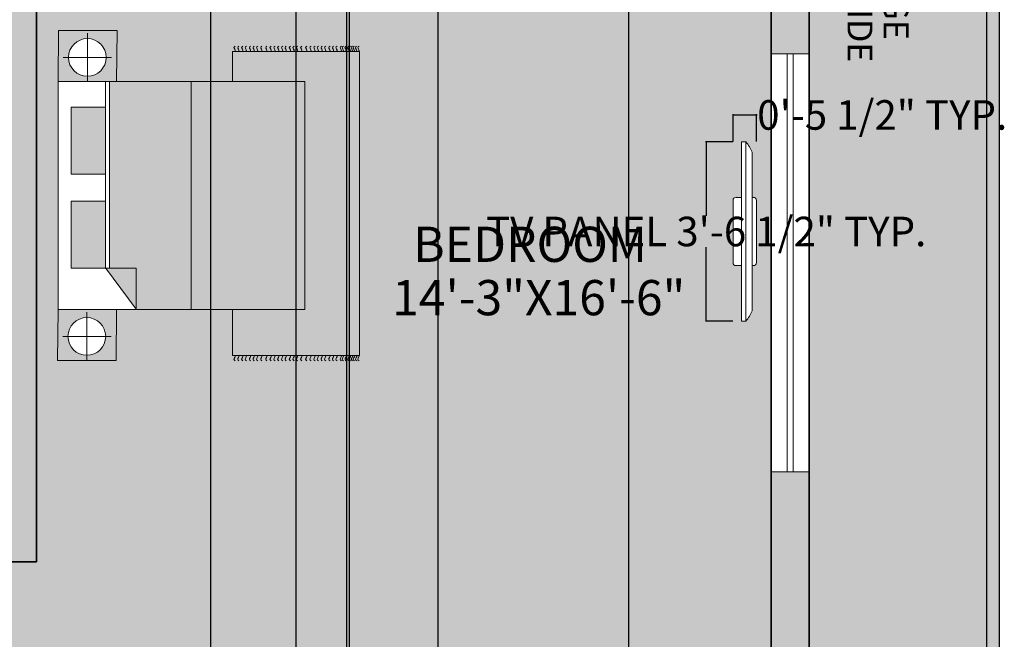
# Model space of a CAD drawing. Units: inches. Extents: x 1884 to 2398, y 474 to 1488.
# Tile 37 of 39: x 2165 to 2398, y 1087 to 1233. Entities that reach past the tile are written whole.
import ezdxf

# ---------------------------------------------------------------- set-up
doc = ezdxf.new("R2010")
doc.units = ezdxf.units.IN
doc.header["$MEASUREMENT"] = 0
for name, color, linetype, lineweight in [('A-ANNO-DIMS', 2, 'Continuous', 18), ('A-AREA-IDEN', 7, 'Continuous', 18), ('A-EQPM', 8, 'Continuous', 18), ('A-FLOR-PATT', 254, 'Continuous', 13), ('A-FURN-PATT', 253, 'Continuous', 13), ('A-WALL-PATT', 250, 'Continuous', 13), ('C-PROP', 7, 'Continuous', 30), ('furniture', 8, 'Continuous', 18), ('walls', 7, 'Continuous', 35), ('windows', 4, 'Continuous', 18)]:
    doc.layers.add(name, color=color, linetype=linetype, lineweight=lineweight)
doc.layers.add('A-FLOR-CASE-PATT', color=251, linetype='Continuous', lineweight=13, true_color=0x636466)
doc.layers.add('L-PVMT-PATT', color=9, linetype='Continuous', lineweight=13, true_color=0xc7c8ca)
doc.styles.get("Standard").update_dxf_attribs({"font": 'arial.ttf'})
doc.dimstyles.get("Standard").update_dxf_attribs({"dimtxt": 7, "dimasz": 0.18, "dimexe": 0.18, "dimexo": 0.0625, "dimgap": 0.09, "dimtad": 0, "dimtih": 1, "dimtoh": 1, "dimzin": 0, "dimdsep": 46, "dimlunit": 3, "dimtxsty": 'Standard', "dimcen": 0.09, "dimadec": 0, "dimazin": 0, "dimtfac": 1, "dimtofl": 0, "dimtmove": 0, "dimatfit": 3, "dimfxl": 1, "dimtolj": 1, "dimtzin": 0, "dimarcsym": 0})

# ---------------------------------------------------------------- blocks, each defined once
blk = doc.blocks.new('PLASMA-LARGE')
at = {"layer": 'furniture'}
for p, q in [((-7.26, 0), (7.26, 0)), ((-18.61, -1), (18.61, -1)), ((-8, -1), (-8, -0.74)), ((8, -1), (8, -0.74)), ((-21, -2.5), (21, -2.5)), ((-21, -2.5), (-21, -3.5)), ((-21, -3.5), (21, -3.5)), ((-8, -3.5), (-8, -4.76)), ((8, -3.5), (8, -4.76)), ((21, -2.5), (21, -3.5)), ((-7.26, -5.5), (7.26, -5.5))]:
    blk.add_line(p, q, dxfattribs=at)
for centre, radius, start, end in [((-7.26, -0.74), 0.744, 90, 180), ((7.26, -0.74), 0.744, 0, 90), ((-13.97, -11.05), 11.07, 114.7602, 129.4175), ((13.97, -11.05), 11.07, 50.5825, 65.2398), ((-7.26, -4.76), 0.744, 180, 270), ((7.26, -4.76), 0.744, 270, 0)]:
    blk.add_arc(centre, radius, start, end, dxfattribs=at)
blk = doc.blocks.new('CARPET')
at = {"layer": 'furniture'}
for p, q in [((-51.53, -98.11), (-51.53, -55.12)), ((-51.53, -55.12), (-41.27, -55.12)), ((36, -55.12), (51.55, -55.12)), ((51.55, -55.12), (51.55, -98.11)), ((51.55, -98.11), (-51.53, -98.11))]:
    blk.add_line(p, q, dxfattribs=at)
for points, knots in [([(-53.37, -55.99), (-53.22, -55.8), (-52.9, -55.41), (-52.34, -55.8), (-51.89, -56.08), (-51.65, -55.91), (-51.53, -55.83)], [0, 0, 0, 0, 0.653278, 1.290138, 1.740457, 2.114451, 2.114451, 2.114451, 2.114451]), ([(53.37, -55.99), (53.22, -55.8), (52.9, -55.41), (52.34, -55.8), (51.89, -56.08), (51.65, -55.91), (51.53, -55.83)], [0, 0, 0, 0, 0.653278, 1.290138, 1.740457, 2.114451, 2.114451, 2.114451, 2.114451]), ([(-53.37, -57.26), (-53.22, -57.07), (-52.9, -56.67), (-52.34, -57.07), (-51.89, -57.35), (-51.65, -57.17), (-51.53, -57.1)], [0, 0, 0, 0, 0.653278, 1.290138, 1.740457, 2.114451, 2.114451, 2.114451, 2.114451]), ([(-53.37, -58.59), (-53.22, -58.4), (-52.9, -58.01), (-52.34, -58.4), (-51.89, -58.68), (-51.65, -58.5), (-51.53, -58.43)], [0, 0, 0, 0, 0.653278, 1.290138, 1.740457, 2.114451, 2.114451, 2.114451, 2.114451]), ([(-53.37, -59.78), (-53.22, -59.58), (-52.9, -59.19), (-52.34, -59.58), (-51.89, -59.86), (-51.65, -59.69), (-51.53, -59.61)], [0, 0, 0, 0, 0.653278, 1.290138, 1.740457, 2.114451, 2.114451, 2.114451, 2.114451]), ([(53.37, -57.26), (53.22, -57.07), (52.9, -56.67), (52.34, -57.07), (51.89, -57.35), (51.65, -57.17), (51.53, -57.1)], [0, 0, 0, 0, 0.653278, 1.290138, 1.740457, 2.114451, 2.114451, 2.114451, 2.114451]), ([(53.37, -58.59), (53.22, -58.4), (52.9, -58.01), (52.34, -58.4), (51.89, -58.68), (51.65, -58.5), (51.53, -58.43)], [0, 0, 0, 0, 0.653278, 1.290138, 1.740457, 2.114451, 2.114451, 2.114451, 2.114451]), ([(53.37, -59.78), (53.22, -59.58), (52.9, -59.19), (52.34, -59.58), (51.89, -59.86), (51.65, -59.69), (51.53, -59.61)], [0, 0, 0, 0, 0.653278, 1.290138, 1.740457, 2.114451, 2.114451, 2.114451, 2.114451]), ([(-53.37, -61.22), (-53.22, -61.02), (-52.9, -60.63), (-52.34, -61.02), (-51.89, -61.3), (-51.65, -61.13), (-51.53, -61.05)], [0, 0, 0, 0, 0.653278, 1.290138, 1.740457, 2.114451, 2.114451, 2.114451, 2.114451]), ([(-53.37, -62.44), (-53.22, -62.25), (-52.9, -61.86), (-52.34, -62.25), (-51.89, -62.53), (-51.65, -62.36), (-51.53, -62.28)], [0, 0, 0, 0, 0.653278, 1.290138, 1.740457, 2.114451, 2.114451, 2.114451, 2.114451]), ([(-53.37, -63.63), (-53.22, -63.43), (-52.9, -63.04), (-52.34, -63.43), (-51.89, -63.72), (-51.65, -63.54), (-51.53, -63.46)], [0, 0, 0, 0, 0.653278, 1.290138, 1.740457, 2.114451, 2.114451, 2.114451, 2.114451]), ([(53.37, -61.22), (53.22, -61.02), (52.9, -60.63), (52.34, -61.02), (51.89, -61.3), (51.65, -61.13), (51.53, -61.05)], [0, 0, 0, 0, 0.653278, 1.290138, 1.740457, 2.114451, 2.114451, 2.114451, 2.114451]), ([(53.37, -62.44), (53.22, -62.25), (52.9, -61.86), (52.34, -62.25), (51.89, -62.53), (51.65, -62.36), (51.53, -62.28)], [0, 0, 0, 0, 0.653278, 1.290138, 1.740457, 2.114451, 2.114451, 2.114451, 2.114451]), ([(53.37, -63.63), (53.22, -63.43), (52.9, -63.04), (52.34, -63.43), (51.89, -63.72), (51.65, -63.54), (51.53, -63.46)], [0, 0, 0, 0, 0.653278, 1.290138, 1.740457, 2.114451, 2.114451, 2.114451, 2.114451]), ([(-53.37, -65.07), (-53.22, -64.87), (-52.9, -64.48), (-52.34, -64.87), (-51.89, -65.15), (-51.65, -64.98), (-51.53, -64.9)], [0, 0, 0, 0, 0.653278, 1.290138, 1.740457, 2.114451, 2.114451, 2.114451, 2.114451]), ([(-53.37, -66.76), (-53.22, -66.56), (-52.9, -66.17), (-52.34, -66.56), (-51.89, -66.84), (-51.65, -66.67), (-51.53, -66.59)], [0, 0, 0, 0, 0.653278, 1.290138, 1.740457, 2.114451, 2.114451, 2.114451, 2.114451]), ([(53.37, -65.07), (53.22, -64.87), (52.9, -64.48), (52.34, -64.87), (51.89, -65.15), (51.65, -64.98), (51.53, -64.9)], [0, 0, 0, 0, 0.653278, 1.290138, 1.740457, 2.114451, 2.114451, 2.114451, 2.114451]), ([(53.37, -66.76), (53.22, -66.56), (52.9, -66.17), (52.34, -66.56), (51.89, -66.84), (51.65, -66.67), (51.53, -66.59)], [0, 0, 0, 0, 0.653278, 1.290138, 1.740457, 2.114451, 2.114451, 2.114451, 2.114451]), ([(-53.37, -68.2), (-53.22, -68), (-52.9, -67.61), (-52.34, -68), (-51.89, -68.28), (-51.65, -68.11), (-51.53, -68.03)], [0, 0, 0, 0, 0.653278, 1.290138, 1.740457, 2.114451, 2.114451, 2.114451, 2.114451]), ([(-53.37, -69.53), (-53.22, -69.33), (-52.9, -68.94), (-52.34, -69.33), (-51.89, -69.61), (-51.65, -69.44), (-51.53, -69.36)], [0, 0, 0, 0, 0.653278, 1.290138, 1.740457, 2.114451, 2.114451, 2.114451, 2.114451]), ([(53.37, -68.2), (53.22, -68), (52.9, -67.61), (52.34, -68), (51.89, -68.28), (51.65, -68.11), (51.53, -68.03)], [0, 0, 0, 0, 0.653278, 1.290138, 1.740457, 2.114451, 2.114451, 2.114451, 2.114451]), ([(53.37, -69.53), (53.22, -69.33), (52.9, -68.94), (52.34, -69.33), (51.89, -69.61), (51.65, -69.44), (51.53, -69.36)], [0, 0, 0, 0, 0.653278, 1.290138, 1.740457, 2.114451, 2.114451, 2.114451, 2.114451]), ([(-53.37, -70.79), (-53.22, -70.6), (-52.9, -70.21), (-52.34, -70.6), (-51.89, -70.88), (-51.65, -70.7), (-51.53, -70.63)], [0, 0, 0, 0, 0.653278, 1.290138, 1.740457, 2.114451, 2.114451, 2.114451, 2.114451]), ([(-53.37, -72.12), (-53.22, -71.93), (-52.9, -71.54), (-52.34, -71.93), (-51.89, -72.21), (-51.65, -72.04), (-51.53, -71.96)], [0, 0, 0, 0, 0.653278, 1.290138, 1.740457, 2.114451, 2.114451, 2.114451, 2.114451]), ([(-53.37, -73.31), (-53.22, -73.11), (-52.9, -72.72), (-52.34, -73.11), (-51.89, -73.4), (-51.65, -73.22), (-51.53, -73.14)], [0, 0, 0, 0, 0.653278, 1.290138, 1.740457, 2.114451, 2.114451, 2.114451, 2.114451]), ([(53.37, -70.79), (53.22, -70.6), (52.9, -70.21), (52.34, -70.6), (51.89, -70.88), (51.65, -70.7), (51.53, -70.63)], [0, 0, 0, 0, 0.653278, 1.290138, 1.740457, 2.114451, 2.114451, 2.114451, 2.114451]), ([(53.37, -72.12), (53.22, -71.93), (52.9, -71.54), (52.34, -71.93), (51.89, -72.21), (51.65, -72.04), (51.53, -71.96)], [0, 0, 0, 0, 0.653278, 1.290138, 1.740457, 2.114451, 2.114451, 2.114451, 2.114451]), ([(53.37, -73.31), (53.22, -73.11), (52.9, -72.72), (52.34, -73.11), (51.89, -73.4), (51.65, -73.22), (51.53, -73.14)], [0, 0, 0, 0, 0.653278, 1.290138, 1.740457, 2.114451, 2.114451, 2.114451, 2.114451]), ([(-53.37, -74.75), (-53.22, -74.55), (-52.9, -74.16), (-52.34, -74.55), (-51.89, -74.83), (-51.65, -74.66), (-51.53, -74.58)], [0, 0, 0, 0, 0.653278, 1.290138, 1.740457, 2.114451, 2.114451, 2.114451, 2.114451]), ([(-53.37, -75.98), (-53.22, -75.78), (-52.9, -75.39), (-52.34, -75.78), (-51.89, -76.06), (-51.65, -75.89), (-51.53, -75.81)], [0, 0, 0, 0, 0.653278, 1.290138, 1.740457, 2.114451, 2.114451, 2.114451, 2.114451]), ([(-53.37, -77.16), (-53.22, -76.96), (-52.9, -76.57), (-52.34, -76.96), (-51.89, -77.25), (-51.65, -77.07), (-51.53, -76.99)], [0, 0, 0, 0, 0.653278, 1.290138, 1.740457, 2.114451, 2.114451, 2.114451, 2.114451]), ([(53.37, -74.75), (53.22, -74.55), (52.9, -74.16), (52.34, -74.55), (51.89, -74.83), (51.65, -74.66), (51.53, -74.58)], [0, 0, 0, 0, 0.653278, 1.290138, 1.740457, 2.114451, 2.114451, 2.114451, 2.114451]), ([(53.37, -75.98), (53.22, -75.78), (52.9, -75.39), (52.34, -75.78), (51.89, -76.06), (51.65, -75.89), (51.53, -75.81)], [0, 0, 0, 0, 0.653278, 1.290138, 1.740457, 2.114451, 2.114451, 2.114451, 2.114451]), ([(53.37, -77.16), (53.22, -76.96), (52.9, -76.57), (52.34, -76.96), (51.89, -77.25), (51.65, -77.07), (51.53, -76.99)], [0, 0, 0, 0, 0.653278, 1.290138, 1.740457, 2.114451, 2.114451, 2.114451, 2.114451]), ([(-53.37, -78.6), (-53.22, -78.4), (-52.9, -78.01), (-52.34, -78.4), (-51.89, -78.68), (-51.65, -78.51), (-51.53, -78.43)], [0, 0, 0, 0, 0.653278, 1.290138, 1.740457, 2.114451, 2.114451, 2.114451, 2.114451]), ([(-53.37, -80.29), (-53.22, -80.09), (-52.9, -79.7), (-52.34, -80.09), (-51.89, -80.37), (-51.65, -80.2), (-51.53, -80.12)], [0, 0, 0, 0, 0.653278, 1.290138, 1.740457, 2.114451, 2.114451, 2.114451, 2.114451]), ([(53.37, -78.6), (53.22, -78.4), (52.9, -78.01), (52.34, -78.4), (51.89, -78.68), (51.65, -78.51), (51.53, -78.43)], [0, 0, 0, 0, 0.653278, 1.290138, 1.740457, 2.114451, 2.114451, 2.114451, 2.114451]), ([(53.37, -80.29), (53.22, -80.09), (52.9, -79.7), (52.34, -80.09), (51.89, -80.37), (51.65, -80.2), (51.53, -80.12)], [0, 0, 0, 0, 0.653278, 1.290138, 1.740457, 2.114451, 2.114451, 2.114451, 2.114451]), ([(-53.37, -81.73), (-53.22, -81.53), (-52.9, -81.14), (-52.34, -81.53), (-51.89, -81.81), (-51.65, -81.64), (-51.53, -81.56)], [0, 0, 0, 0, 0.653278, 1.290138, 1.740457, 2.114451, 2.114451, 2.114451, 2.114451]), ([(-53.37, -83.06), (-53.22, -82.86), (-52.9, -82.47), (-52.34, -82.86), (-51.89, -83.14), (-51.65, -82.97), (-51.53, -82.89)], [0, 0, 0, 0, 0.653278, 1.290138, 1.740457, 2.114451, 2.114451, 2.114451, 2.114451]), ([(53.37, -81.73), (53.22, -81.53), (52.9, -81.14), (52.34, -81.53), (51.89, -81.81), (51.65, -81.64), (51.53, -81.56)], [0, 0, 0, 0, 0.653278, 1.290138, 1.740457, 2.114451, 2.114451, 2.114451, 2.114451]), ([(53.37, -83.06), (53.22, -82.86), (52.9, -82.47), (52.34, -82.86), (51.89, -83.14), (51.65, -82.97), (51.53, -82.89)], [0, 0, 0, 0, 0.653278, 1.290138, 1.740457, 2.114451, 2.114451, 2.114451, 2.114451]), ([(-53.37, -84.18), (-53.22, -83.99), (-52.9, -83.6), (-52.34, -83.99), (-51.89, -84.27), (-51.65, -84.09), (-51.53, -84.02)], [0, 0, 0, 0, 0.653278, 1.290138, 1.740457, 2.114451, 2.114451, 2.114451, 2.114451]), ([(-53.37, -85.51), (-53.22, -85.32), (-52.9, -84.93), (-52.34, -85.32), (-51.89, -85.6), (-51.65, -85.42), (-51.53, -85.35)], [0, 0, 0, 0, 0.653278, 1.290138, 1.740457, 2.114451, 2.114451, 2.114451, 2.114451]), ([(-53.37, -86.7), (-53.22, -86.5), (-52.9, -86.11), (-52.34, -86.5), (-51.89, -86.78), (-51.65, -86.61), (-51.53, -86.53)], [0, 0, 0, 0, 0.653278, 1.290138, 1.740457, 2.114451, 2.114451, 2.114451, 2.114451]), ([(53.37, -84.18), (53.22, -83.99), (52.9, -83.6), (52.34, -83.99), (51.89, -84.27), (51.65, -84.09), (51.53, -84.02)], [0, 0, 0, 0, 0.653278, 1.290138, 1.740457, 2.114451, 2.114451, 2.114451, 2.114451]), ([(53.37, -85.51), (53.22, -85.32), (52.9, -84.93), (52.34, -85.32), (51.89, -85.6), (51.65, -85.42), (51.53, -85.35)], [0, 0, 0, 0, 0.653278, 1.290138, 1.740457, 2.114451, 2.114451, 2.114451, 2.114451]), ([(53.37, -86.7), (53.22, -86.5), (52.9, -86.11), (52.34, -86.5), (51.89, -86.78), (51.65, -86.61), (51.53, -86.53)], [0, 0, 0, 0, 0.653278, 1.290138, 1.740457, 2.114451, 2.114451, 2.114451, 2.114451]), ([(-53.37, -88.14), (-53.22, -87.94), (-52.9, -87.55), (-52.34, -87.94), (-51.89, -88.22), (-51.65, -88.05), (-51.53, -87.97)], [0, 0, 0, 0, 0.653278, 1.290138, 1.740457, 2.114451, 2.114451, 2.114451, 2.114451]), ([(-53.37, -89.36), (-53.22, -89.17), (-52.9, -88.78), (-52.34, -89.17), (-51.89, -89.45), (-51.65, -89.28), (-51.53, -89.2)], [0, 0, 0, 0, 0.653278, 1.290138, 1.740457, 2.114451, 2.114451, 2.114451, 2.114451]), ([(-53.37, -90.55), (-53.22, -90.35), (-52.9, -89.96), (-52.34, -90.35), (-51.89, -90.64), (-51.65, -90.46), (-51.53, -90.38)], [0, 0, 0, 0, 0.653278, 1.290138, 1.740457, 2.114451, 2.114451, 2.114451, 2.114451]), ([(53.37, -88.14), (53.22, -87.94), (52.9, -87.55), (52.34, -87.94), (51.89, -88.22), (51.65, -88.05), (51.53, -87.97)], [0, 0, 0, 0, 0.653278, 1.290138, 1.740457, 2.114451, 2.114451, 2.114451, 2.114451]), ([(53.37, -89.36), (53.22, -89.17), (52.9, -88.78), (52.34, -89.17), (51.89, -89.45), (51.65, -89.28), (51.53, -89.2)], [0, 0, 0, 0, 0.653278, 1.290138, 1.740457, 2.114451, 2.114451, 2.114451, 2.114451]), ([(53.37, -90.55), (53.22, -90.35), (52.9, -89.96), (52.34, -90.35), (51.9, -90.63), (51.66, -90.47), (51.55, -90.4)], [0, 0, 0, 0, 0.653278, 1.290138, 1.740457, 2.0926, 2.0926, 2.0926, 2.0926]), ([(-53.37, -91.99), (-53.22, -91.79), (-52.9, -91.4), (-52.34, -91.79), (-51.89, -92.07), (-51.65, -91.9), (-51.53, -91.82)], [0, 0, 0, 0, 0.653278, 1.290138, 1.740457, 2.114451, 2.114451, 2.114451, 2.114451]), ([(-53.37, -92.69), (-53.22, -92.48), (-52.9, -92.08), (-52.35, -92.49), (-51.89, -92.77), (-51.65, -92.6), (-51.53, -92.52)], [0, 0, 0, 0, 0.663904, 1.307406, 1.757725, 2.131719, 2.131719, 2.131719, 2.131719]), ([(-53.37, -93.61), (-53.22, -93.42), (-52.9, -93.03), (-52.34, -93.42), (-51.89, -93.7), (-51.65, -93.52), (-51.53, -93.45)], [0, 0, 0, 0, 0.653278, 1.290138, 1.740457, 2.114451, 2.114451, 2.114451, 2.114451]), ([(53.37, -91.99), (53.22, -91.79), (52.9, -91.4), (52.34, -91.79), (51.9, -92.07), (51.66, -91.91), (51.55, -91.83)], [0, 0, 0, 0, 0.653278, 1.290138, 1.740457, 2.0926, 2.0926, 2.0926, 2.0926]), ([(53.37, -92.69), (53.22, -92.49), (52.9, -92.09), (52.34, -92.49), (51.9, -92.77), (51.66, -92.61), (51.55, -92.53)], [0, 0, 0, 0, 0.656792, 1.295826, 1.746145, 2.098292, 2.098292, 2.098292, 2.098292]), ([(53.37, -93.66), (53.22, -93.46), (52.9, -93.07), (52.34, -93.46), (51.9, -93.74), (51.66, -93.58), (51.55, -93.5)], [0, 0, 0, 0, 0.653278, 1.290138, 1.740457, 2.0926, 2.0926, 2.0926, 2.0926]), ([(-53.37, -94.55), (-53.22, -94.35), (-52.9, -93.96), (-52.34, -94.35), (-51.89, -94.63), (-51.65, -94.46), (-51.53, -94.38)], [0, 0, 0, 0, 0.653278, 1.290138, 1.740457, 2.114451, 2.114451, 2.114451, 2.114451]), ([(-53.37, -95.05), (-53.22, -94.85), (-52.9, -94.46), (-52.34, -94.85), (-51.89, -95.14), (-51.65, -94.96), (-51.53, -94.88)], [0, 0, 0, 0, 0.653278, 1.290138, 1.740457, 2.114451, 2.114451, 2.114451, 2.114451]), ([(-53.37, -95.73), (-53.22, -95.54), (-52.9, -95.15), (-52.34, -95.54), (-51.89, -95.82), (-51.65, -95.65), (-51.53, -95.57)], [0, 0, 0, 0, 0.653278, 1.290138, 1.740457, 2.114451, 2.114451, 2.114451, 2.114451]), ([(-53.37, -96.38), (-53.22, -96.18), (-52.9, -95.79), (-52.34, -96.18), (-51.89, -96.47), (-51.65, -96.29), (-51.53, -96.21)], [0, 0, 0, 0, 0.653278, 1.290138, 1.740457, 2.114451, 2.114451, 2.114451, 2.114451]), ([(-53.37, -97.17), (-53.22, -96.98), (-52.9, -96.59), (-52.34, -96.98), (-51.89, -97.26), (-51.65, -97.08), (-51.53, -97.01)], [0, 0, 0, 0, 0.653278, 1.290138, 1.740457, 2.114451, 2.114451, 2.114451, 2.114451]), ([(53.37, -95.78), (53.22, -95.58), (52.9, -95.19), (52.34, -95.58), (51.89, -95.86), (51.65, -95.69), (51.53, -95.61)], [0, 0, 0, 0, 0.653278, 1.290138, 1.740457, 2.114451, 2.114451, 2.114451, 2.114451]), ([(53.37, -96.43), (53.22, -96.23), (52.9, -95.84), (52.34, -96.23), (51.89, -96.51), (51.65, -96.34), (51.53, -96.26)], [0, 0, 0, 0, 0.653278, 1.290138, 1.740457, 2.114451, 2.114451, 2.114451, 2.114451]), ([(53.37, -97.22), (53.22, -97.02), (52.9, -96.63), (52.34, -97.02), (51.89, -97.3), (51.65, -97.13), (51.53, -97.05)], [0, 0, 0, 0, 0.653278, 1.290138, 1.740457, 2.114451, 2.114451, 2.114451, 2.114451]), ([(53.37, -94.59), (53.22, -94.4), (52.9, -94.01), (52.34, -94.4), (51.9, -94.68), (51.66, -94.51), (51.55, -94.44)], [0, 0, 0, 0, 0.653278, 1.290138, 1.740457, 2.0926, 2.0926, 2.0926, 2.0926]), ([(53.37, -95.1), (53.22, -94.9), (52.9, -94.51), (52.34, -94.9), (51.9, -95.18), (51.66, -95.02), (51.55, -94.94)], [0, 0, 0, 0, 0.653278, 1.290138, 1.740457, 2.0926, 2.0926, 2.0926, 2.0926]), ([(-53.37, -97.99), (-53.22, -97.79), (-52.9, -97.4), (-52.34, -97.79), (-51.89, -98.08), (-51.65, -97.9), (-51.53, -97.82)], [0, 0, 0, 0, 0.653278, 1.290138, 1.740457, 2.114451, 2.114451, 2.114451, 2.114451]), ([(53.37, -97.99), (53.22, -97.79), (52.9, -97.4), (52.34, -97.79), (51.89, -98.08), (51.65, -97.9), (51.53, -97.82)], [0, 0, 0, 0, 0.653278, 1.290138, 1.740457, 2.114451, 2.114451, 2.114451, 2.114451])]:
    blk.add_open_spline(points, degree=3, knots=knots, dxfattribs=at)
blk = doc.blocks.new('A$C58D270C6')
at = {"layer": 'furniture'}
for p, q in [((9.09, 124.13), (9.09, 108.87)), ((1.46, 116.5), (16.73, 116.5)), ((14.97, 94.84), (24.62, 107.92)), ((24.62, 94.93), (24.62, 107.92)), ((42.08, 108), (42.08, 36)), ((14.97, 94.93), (24.62, 94.93)), ((14.97, 94.84), (14.97, 36)), ((16.22, 94.93), (16.22, 36)), ((9.25, 36), (9.25, 20.74)), ((1.62, 28.37), (16.88, 28.37))]:
    blk.add_line(p, q, dxfattribs=at)
for points in [[(18.5, 108), (18.34, 124.13), (-0.16, 124.13), (0, 108)], [(0, 108), (77.91, 108), (77.91, 36), (0, 36)], [(4.09, 94.93), (14.97, 94.93), (14.97, 73.83), (4.09, 73.83)], [(4.09, 65.23), (14.97, 65.23), (14.97, 44.13), (4.09, 44.13)], [(18.65, 19.87), (18.5, 36), (0, 36), (0.16, 19.87)]]:
    blk.add_lwpolyline(points, close=True, dxfattribs=at)
for centre in [(9.09, 116.5), (9.25, 28.37)]:
    blk.add_circle(centre, 5.95, dxfattribs=at)
at = {"layer": 'furniture', "xscale": 0.9312884925094044, "yscale": 0.9312884925094044, "zscale": 0.9312884925094044, "rotation": 90}
blk.add_blockref('CARPET', (3.79, 74.47), dxfattribs=at)
blk = doc.blocks.new('*D27')
at = {"layer": 'A-ANNO-DIMS', "color": 0, "lineweight": -2, "transparency": 16777216}
for p, q in [((2333.47, 1204.46), (2326.98, 1204.46)), ((2327.16, 1204.28), (2327.16, 1186.93)), ((2327.16, 1162.17), (2327.16, 1179.51)), ((2333.47, 1161.99), (2326.98, 1161.99))]:
    blk.add_line(p, q, dxfattribs=at)
at = {"layer": 'A-ANNO-DIMS', "color": 0, "lineweight": 100, "transparency": 16777216}
for points in [[(2327.13, 1204.28), (2327.19, 1204.28), (2327.16, 1204.46)], [(2327.13, 1162.17), (2327.19, 1162.17), (2327.16, 1161.99)]]:
    blk.add_solid(points, dxfattribs=at)
at = {"layer": 'Defpoints', "color": 0, "lineweight": 100, "transparency": 16777216}
for p in [(2327.16, 1204.46), (2333.53, 1204.46), (2333.53, 1161.99)]:
    blk.add_point(p, dxfattribs=at)
at = {"layer": 'A-ANNO-DIMS', "color": 0, "transparency": 16777216, "insert": (2327.16, 1183.22), "char_height": 7, "attachment_point": 5}
blk.add_mtext('\\A1;TV PANEL 3\'-6 1/2" TYP.', dxfattribs=at)
blk = doc.blocks.new('*D28')
at = {"layer": 'A-ANNO-DIMS', "color": 0, "lineweight": -2, "transparency": 16777216}
for p, q in [((2333.53, 1204.52), (2333.53, 1211.01)), ((2333.71, 1210.83), (2338.91, 1210.83)), ((2339.09, 1204.52), (2339.09, 1211.01)), ((2339.09, 1210.83), (2339.27, 1210.83))]:
    blk.add_line(p, q, dxfattribs=at)
at = {"layer": 'A-ANNO-DIMS', "color": 0, "lineweight": 100, "transparency": 16777216}
for points in [[(2333.71, 1210.86), (2333.71, 1210.8), (2333.53, 1210.83)], [(2338.91, 1210.86), (2338.91, 1210.8), (2339.09, 1210.83)]]:
    blk.add_solid(points, dxfattribs=at)
at = {"layer": 'Defpoints', "color": 0, "lineweight": 100, "transparency": 16777216}
for p in [(2339.09, 1210.83), (2333.53, 1204.46), (2339.09, 1204.46)]:
    blk.add_point(p, dxfattribs=at)
at = {"layer": 'A-ANNO-DIMS', "color": 0, "transparency": 16777216, "insert": (2368.85, 1210.83), "char_height": 7, "attachment_point": 5}
blk.add_mtext('\\A1;0\'-5 1/2" TYP.', dxfattribs=at)
blk = doc.blocks.new('*D44')
at = {"layer": 'A-ANNO-DIMS', "color": 0, "lineweight": -2, "transparency": 16777216}
for p, q in [((2209.76, 1247.82), (2209.76, 484)), ((2230.03, 1247.82), (2230.03, 484)), ((2209.94, 484.18), (2229.85, 484.18)), ((2230.03, 484.18), (2230.21, 484.18))]:
    blk.add_line(p, q, dxfattribs=at)
at = {"layer": 'A-ANNO-DIMS', "color": 0, "lineweight": 100, "transparency": 16777216}
for points in [[(2209.94, 484.21), (2209.94, 484.15), (2209.76, 484.18)], [(2229.85, 484.21), (2229.85, 484.15), (2230.03, 484.18)]]:
    blk.add_solid(points, dxfattribs=at)
at = {"layer": 'Defpoints', "color": 0, "lineweight": 100, "transparency": 16777216}
for p in [(2209.76, 1247.88), (2230.03, 1247.88), (2230.03, 484.18)]:
    blk.add_point(p, dxfattribs=at)
at = {"layer": 'A-ANNO-DIMS', "color": 0, "transparency": 16777216, "insert": (2247.43, 484.18), "char_height": 7, "attachment_point": 5}
blk.add_mtext('\\A1;1\'-8 1/2"', dxfattribs=at)
blk = doc.blocks.new('*D45')
at = {"layer": 'A-ANNO-DIMS', "color": 0, "lineweight": -2, "transparency": 16777216}
for p, q in [((2242.62, 1322.82), (2242.62, 484)), ((2263.62, 1322.82), (2263.62, 484)), ((2242.8, 484.18), (2244.05, 484.18)), ((2263.44, 484.18), (2262.18, 484.18))]:
    blk.add_line(p, q, dxfattribs=at)
at = {"layer": 'A-ANNO-DIMS', "color": 0, "lineweight": 100, "transparency": 16777216}
for points in [[(2242.8, 484.21), (2242.8, 484.15), (2242.62, 484.18)], [(2263.44, 484.21), (2263.44, 484.15), (2263.62, 484.18)]]:
    blk.add_solid(points, dxfattribs=at)
at = {"layer": 'Defpoints', "color": 0, "lineweight": 100, "transparency": 16777216}
for p in [(2242.62, 1322.88), (2263.62, 1322.88), (2263.62, 484.18)]:
    blk.add_point(p, dxfattribs=at)
at = {"layer": 'A-ANNO-DIMS', "color": 0, "transparency": 16777216, "insert": (2253.12, 484.18), "char_height": 7, "attachment_point": 5}
blk.add_mtext('\\A1;1\'-9"', dxfattribs=at)
blk = doc.blocks.new('*D52')
at = {"layer": 'A-ANNO-DIMS', "color": 0, "lineweight": -2, "transparency": 16777216}
for p, q in [((2308.85, 820.89), (2308.85, 1477.76)), ((2309.03, 1477.58), (2342.35, 1477.58)), ((2342.53, 820.89), (2342.53, 1477.76)), ((2342.53, 1477.58), (2342.71, 1477.58))]:
    blk.add_line(p, q, dxfattribs=at)
at = {"layer": 'A-ANNO-DIMS', "color": 0, "lineweight": 100, "transparency": 16777216}
for points in [[(2309.03, 1477.61), (2309.03, 1477.55), (2308.85, 1477.58)], [(2342.35, 1477.61), (2342.35, 1477.55), (2342.53, 1477.58)]]:
    blk.add_solid(points, dxfattribs=at)
at = {"layer": 'Defpoints', "color": 0, "lineweight": 100, "transparency": 16777216}
for p in [(2342.53, 1477.58), (2308.85, 820.83), (2342.53, 820.83)]:
    blk.add_point(p, dxfattribs=at)
at = {"layer": 'A-ANNO-DIMS', "color": 0, "transparency": 16777216, "insert": (2360.32, 1477.58), "char_height": 7, "attachment_point": 5}
blk.add_mtext('\\A1;2\'-9 1/2"', dxfattribs=at)
blk = doc.blocks.new('*D54')
at = {"layer": 'A-ANNO-DIMS', "color": 0, "lineweight": -2, "transparency": 16777216}
for p, q in [((2242.06, 893.03), (2242.06, 1477.76)), ((2242.24, 1477.58), (2266.06, 1477.58)), ((2308.67, 1477.58), (2284.85, 1477.58)), ((2308.85, 893.03), (2308.85, 1477.76))]:
    blk.add_line(p, q, dxfattribs=at)
at = {"layer": 'A-ANNO-DIMS', "color": 0, "lineweight": 100, "transparency": 16777216}
for points in [[(2242.24, 1477.61), (2242.24, 1477.55), (2242.06, 1477.58)], [(2308.67, 1477.61), (2308.67, 1477.55), (2308.85, 1477.58)]]:
    blk.add_solid(points, dxfattribs=at)
at = {"layer": 'Defpoints', "color": 0, "lineweight": 100, "transparency": 16777216}
for p in [(2308.85, 1477.58), (2242.06, 892.97), (2308.85, 892.97)]:
    blk.add_point(p, dxfattribs=at)
at = {"layer": 'A-ANNO-DIMS', "color": 0, "transparency": 16777216, "insert": (2275.45, 1477.58), "char_height": 7, "attachment_point": 5}
blk.add_mtext('\\A1;5\'-7"', dxfattribs=at)

msp = doc.modelspace()

# ---------------------------------------------------------------- hatches: boundary and pattern name
at = {"layer": 'A-FLOR-CASE-PATT'}
h = msp.add_hatch(color=256, dxfattribs=at)
h.dxf.hatch_style = 1
h.paths.add_polyline_path([(2326.148, 1214.404), (2341.045, 1214.404), (2341.045, 1149.961), (2326.148, 1149.961)])
h.paths.add_polyline_path([(2335.555, 1161.985), (2336.567, 1161.985, 0.0640419), (2338.083, 1164.405), (2338.083, 1175.132), (2338.342, 1175.132, 0.4142136), (2339.095, 1175.885), (2339.095, 1190.56, 0.4142136), (2338.342, 1191.313), (2338.083, 1191.313), (2338.083, 1202.04, 0.0640419), (2336.567, 1204.46), (2335.555, 1204.46), (2335.555, 1191.313), (2334.285, 1191.313, 0.4142136), (2333.533, 1190.56), (2333.533, 1175.885, 0.4142136), (2334.285, 1175.132), (2335.555, 1175.132)], flags=16)
at = {"layer": 'A-FLOR-PATT'}
h = msp.add_hatch(color=256, dxfattribs=at)
h.dxf.hatch_style = 1
h.paths.add_polyline_path([(2117.529, 815.801), (2126.529, 815.801), (2126.529, 880.382), (2117.529, 880.382), (2117.529, 892.385), (1961.529, 892.385), (1961.529, 756.915), (1964.529, 756.915), (1964.529, 759.915), (1995.529, 759.915), (1995.529, 753.915), (1972.862, 753.915), (1967.529, 756.915), (1967.529, 654.915), (1972.862, 657.915), (1995.529, 657.915), (1995.529, 651.915), (1964.529, 651.915), (1964.529, 654.915), (1961.529, 654.915), (1961.529, 640.385), (2117.529, 640.385), (2117.529, 646.578), (2126.529, 646.578), (2126.529, 676.183), (2117.529, 676.183)])
h.paths.add_polyline_path([(2012.246, 808.929), (2012.05, 810.185), (2032.542, 810.185), (2032.346, 808.929)], flags=16)
h.paths.add_polyline_path([(2010.381, 820.864), (1994.658, 820.864), (1994.658, 831.561), (1984.608, 833.132), (1984.608, 853.821), (1994.658, 855.391), (1994.658, 866.089), (2010.381, 866.089), (2011.951, 876.139), (2032.64, 876.139), (2034.211, 866.089), (2045.556, 866.089), (2047.127, 876.139), (2067.816, 876.139), (2069.386, 866.089), (2085.109, 866.089), (2085.109, 855.391), (2095.159, 853.821), (2095.159, 833.132), (2085.109, 831.561), (2085.109, 820.864), (2069.386, 820.864), (2067.816, 810.814), (2047.127, 810.814), (2045.556, 820.864), (2034.211, 820.864), (2032.64, 810.814), (2011.951, 810.814)], flags=16)
h.paths.add_polyline_path([(1982.724, 833.426), (1982.724, 853.526), (1983.98, 853.723), (1983.98, 833.23)], flags=16)
h.paths.add_polyline_path([(1994.529, 753.54), (1994.529, 658.29), (1973.529, 658.29), (1973.529, 753.54)], flags=16)
h.paths.add_polyline_path([(2084.486, 843.527), (2084.592, 843.502), (2084.681, 843.487), (2084.813, 843.477), (2084.913, 843.477), (2084.669, 843.482), (2084.336, 843.565), (2084.116, 843.617), (2083.8, 843.686), (2083.105, 843.827), (2082.836, 843.874), (2083.604, 843.729), (2084.206, 843.597)], flags=0)
h.paths.add_polyline_path([(2047.421, 808.929), (2047.225, 810.185), (2067.718, 810.185), (2067.521, 808.929)], flags=16)
h.paths.add_polyline_path([(2066.01, 849.505), (2066.429, 849.687), (2066.798, 849.882), (2067.129, 850.085), (2067.43, 850.293), (2067.711, 850.502), (2068.176, 850.856), (2068.689, 851.205), (2069.305, 851.531), (2070.015, 851.784), (2070.844, 851.944), (2071.081, 851.956), (2070.629, 851.902), (2070.212, 851.822), (2069.827, 851.717), (2069.471, 851.59), (2069.139, 851.443), (2068.828, 851.279), (2068.534, 851.1), (2068.254, 850.909), (2067.983, 850.709), (2067.502, 850.343), (2066.951, 849.962), (2066.224, 849.579)], flags=0)
h.paths.add_polyline_path([(2059.423, 853.221), (2059.827, 853.278), (2060.171, 853.358), (2060.465, 853.463), (2060.714, 853.589), (2060.926, 853.736), (2061.107, 853.902), (2061.258, 854.086), (2061.377, 854.284), (2061.462, 854.495), (2061.514, 854.715), (2061.53, 854.943), (2061.508, 855.176), (2061.449, 855.411), (2061.352, 855.646), (2061.224, 855.882), (2061.07, 856.117), (2060.9, 856.353), (2060.719, 856.588), (2060.406, 856.993), (2060.103, 857.424), (2059.858, 857.888), (2059.691, 858.467), (2059.836, 859.091), (2060.305, 859.532), (2060.844, 859.798), (2061.513, 859.935), (2062.253, 859.905), (2062.483, 859.849), (2062.078, 859.912), (2061.695, 859.928), (2061.336, 859.899), (2061.005, 859.831), (2060.703, 859.729), (2060.437, 859.597), (2060.208, 859.441), (2060.021, 859.265), (2059.879, 859.075), (2059.785, 858.874), (2059.737, 858.664), (2059.73, 858.447), (2059.761, 858.224), (2059.827, 857.996), (2059.923, 857.765), (2060.047, 857.53), (2060.193, 857.295), (2060.359, 857.06), (2060.537, 856.824), (2060.867, 856.399), (2061.171, 855.978), (2061.422, 855.518), (2061.567, 854.943), (2061.41, 854.272), (2060.947, 853.707), (2060.335, 853.397), (2059.649, 853.236)], flags=0)
h.paths.add_polyline_path([(2050.778, 859.745), (2051.07, 859.87), (2051.295, 860.017), (2051.467, 860.183), (2051.594, 860.365), (2051.679, 860.56), (2051.726, 860.763), (2051.739, 860.971), (2051.722, 861.18), (2051.677, 861.387), (2051.609, 861.587), (2051.521, 861.779), (2051.421, 861.962), (2051.312, 862.138), (2051.203, 862.307), (2050.966, 862.68), (2050.793, 863.193), (2051.021, 863.699), (2051.483, 864.018), (2052.09, 864.138), (2052.773, 864.157), (2053.007, 864.142), (2052.603, 864.152), (2052.258, 864.142), (2051.965, 864.113), (2051.716, 864.064), (2051.504, 863.995), (2051.322, 863.907), (2051.17, 863.802), (2051.048, 863.682), (2050.954, 863.55), (2050.891, 863.408), (2050.856, 863.259), (2050.851, 863.105), (2050.876, 862.948), (2050.929, 862.791), (2051.005, 862.633), (2051.098, 862.472), (2051.203, 862.307), (2051.312, 862.138), (2051.556, 861.742), (2051.751, 861.167), (2051.712, 860.535), (2051.398, 860.085), (2050.949, 859.79)], flags=0)
h.paths.add_polyline_path([(2022.768, 719.264), (2050.461, 719.264), (2050.461, 717.226), (2052.426, 717.226), (2052.426, 715.033), (2050.461, 715.033), (2050.461, 703.738), (2022.768, 703.738)], flags=16)
h.paths.add_polyline_path([(2012.246, 878.023), (2032.346, 878.023), (2032.542, 876.767), (2012.05, 876.767)], flags=16)
h.paths.add_polyline_path([(2035.324, 713.103), (2035.342, 713.294), (2035.192, 713.202)], flags=0)
h.paths.add_polyline_path([(2036.484, 711.63), (2036.583, 711.849), (2036.39, 711.898)], flags=0)
h.paths.add_polyline_path([(2036.074, 712.744), (2035.993, 712.481), (2035.724, 712.516), (2035.794, 712.726)], flags=0)
h.paths.add_polyline_path([(2035.846, 710.909), (2035.753, 710.958), (2035.702, 710.88)], flags=0)
h.paths.add_polyline_path([(2037.818, 712.019), (2037.948, 712.06), (2037.987, 712.161), (2037.815, 712.02)], flags=0)
h.paths.add_polyline_path([(2038.451, 709.517), (2038.464, 709.428), (2038.586, 709.442)], flags=0)
h.paths.add_polyline_path([(2037.805, 709.806), (2037.818, 709.807), (2037.804, 709.823)], flags=0)
h.paths.add_polyline_path([(2036.7, 711.245), (2036.698, 711.236), (2036.813, 711.211)], flags=0)
h.paths.add_polyline_path([(2035.928, 708.897), (2035.668, 708.871), (2035.706, 708.667)], flags=0)
h.paths.add_polyline_path([(2036.414, 710.976), (2035.932, 709.859), (2036.792, 710.484), (2036.5, 710.934)], flags=0)
h.paths.add_polyline_path([(2038.298, 712.115), (2038.499, 712.058), (2038.612, 712.269), (2038.39, 712.332)], flags=0)
h.paths.add_polyline_path([(2047.421, 878.023), (2067.521, 878.023), (2067.718, 876.767), (2047.225, 876.767)], flags=16)
h.paths.add_polyline_path([(2049.647, 705.093, -1), (2048.845, 705.093, -1)], flags=0)
h.paths.add_polyline_path([(2095.787, 853.723), (2097.043, 853.526), (2097.043, 833.426), (2095.787, 833.23)], flags=16)
h.paths.add_polyline_path([(2110.739, 745.339), (2111.75, 745.339, -0.0640419), (2113.267, 742.92), (2113.267, 732.192), (2113.526, 732.192, -0.4142136), (2114.278, 731.439), (2114.278, 716.764, -0.4142136), (2113.526, 716.011), (2113.267, 716.011), (2113.267, 705.284, -0.0640419), (2111.75, 702.864), (2110.739, 702.864), (2110.739, 716.011), (2109.469, 716.011, -0.4142136), (2108.716, 716.764), (2108.716, 731.439, -0.4142136), (2109.469, 732.192), (2110.739, 732.192)], flags=16)
h.paths.add_polyline_path([(1998.045, 668.909), (2002.449, 668.909), (2002.449, 652.273), (2002.724, 652.763), (2002.724, 668.175), (2019.972, 668.175), (2019.972, 652.763), (2020.247, 652.273), (2020.247, 668.909), (2024.651, 668.909), (2029.055, 668.909), (2029.055, 652.273), (2029.33, 652.763), (2029.33, 668.175), (2046.578, 668.175), (2046.578, 652.763), (2046.853, 652.273), (2046.853, 668.909), (2051.257, 668.909), (2051.257, 646.157), (2049.055, 646.157), (2049.055, 643.955), (2026.853, 643.955), (2026.853, 646.157), (2024.651, 646.157), (2022.449, 646.157), (2022.449, 643.955), (2000.247, 643.955), (2000.247, 646.157), (1998.045, 646.157)], flags=16)
h.paths.add_polyline_path([(2342.529, 1247.885), (2265.892, 1247.885), (2230.029, 1247.885), (2209.755, 1247.885), (2168.6, 1247.885), (2168.6, 1104.929), (2158.029, 1104.929), (2158.029, 1079.411), (2168.6, 1079.411), (2168.6, 1062.466), (2342.529, 1062.466), (2342.529, 1093.809)])
h.paths.add_polyline_path([(2215.03, 1153.876), (2215.03, 1164.739), (2187.559, 1164.739), (2187.442, 1152.641), (2173.568, 1152.641), (2173.684, 1164.739), (2173.684, 1218.739), (2173.801, 1230.837), (2187.675, 1230.837), (2187.559, 1218.739), (2215.03, 1218.739), (2215.03, 1225.879), (2245.053, 1225.879), (2245.053, 1153.876)], flags=16)
h.paths.add_polyline_path([(2192.147, 1164.797), (2184.963, 1174.54), (2184.915, 1174.54), (2176.755, 1174.54), (2176.755, 1190.363), (2184.915, 1190.363), (2184.915, 1196.819), (2176.755, 1196.819), (2176.755, 1212.641), (2184.915, 1212.641), (2184.915, 1174.606), (2184.963, 1174.54), (2192.147, 1174.54)], flags=0)
h.paths.add_polyline_path([(2184.971, 1158.364, -1), (2176.039, 1158.364, -1)], flags=0)
h.paths.add_polyline_path([(2335.555, 1161.985), (2335.555, 1175.132), (2334.285, 1175.132, -0.4142136), (2333.533, 1175.885), (2333.533, 1190.56, -0.4142136), (2334.285, 1191.313), (2335.555, 1191.313), (2335.555, 1204.46), (2336.567, 1204.46, -0.0640419), (2338.083, 1202.04), (2338.083, 1191.313), (2338.342, 1191.313, -0.4142136), (2339.095, 1190.56), (2339.095, 1175.885, -0.4142136), (2338.342, 1175.132), (2338.083, 1175.132), (2338.083, 1164.405, -0.0640419), (2336.567, 1161.985)], flags=16)
h.paths.add_polyline_path([(2176.155, 1224.462, -1), (2185.087, 1224.462, -1)], flags=0)
h.paths.add_polyline_path([(2158.029, 1276.197), (2158.029, 1322.885), (2148.233, 1322.885), (2092.029, 1322.885), (1961.529, 1322.885), (1961.529, 1166.885), (2116.005, 1166.885), (2116.005, 1157.885), (2152.638, 1157.885), (2152.638, 1166.885), (2158.029, 1166.885)])
h.paths.add_polyline_path([(2006.352, 1204.245), (2006.352, 1215.108), (1978.881, 1215.108), (1978.764, 1203.01), (1964.89, 1203.01), (1965.006, 1215.108), (1965.006, 1269.108), (1965.123, 1281.207), (1978.997, 1281.207), (1978.881, 1269.108), (2006.352, 1269.108), (2006.352, 1276.248), (2036.375, 1276.248), (2036.375, 1204.245)], flags=16)
h.paths.add_polyline_path([(1983.469, 1215.166), (1976.285, 1224.909), (1976.237, 1224.909), (1968.077, 1224.909), (1968.077, 1240.732), (1976.237, 1240.732), (1976.237, 1247.188), (1968.077, 1247.188), (1968.077, 1263.011), (1976.237, 1263.011), (1976.237, 1224.975), (1976.285, 1224.909), (1983.469, 1224.909)], flags=0)
h.paths.add_polyline_path([(1976.293, 1208.733, -1), (1967.361, 1208.733, -1)], flags=0)
h.paths.add_polyline_path([(1967.477, 1274.832, -1), (1976.41, 1274.832, -1)], flags=0)
h.paths.add_polyline_path([(2152.587, 1223.485), (2152.587, 1236.632), (2151.317, 1236.632, -0.4142136), (2150.564, 1237.385), (2150.564, 1252.06, -0.4142136), (2151.317, 1252.813), (2152.587, 1252.813), (2152.587, 1265.959), (2153.598, 1265.959, -0.0640419), (2155.115, 1263.54), (2155.115, 1252.813), (2155.374, 1252.813, -0.4142136), (2156.126, 1252.06), (2156.126, 1237.385, -0.4142136), (2155.374, 1236.632), (2155.115, 1236.632), (2155.115, 1225.904, -0.0640419), (2153.598, 1223.485)], flags=16)
h.paths.add_polyline_path([(2250.676, 1161.101), (2322.077, 1161.101), (2322.077, 1173.886), (2250.676, 1173.886)], flags=24)
h.paths.add_polyline_path([(2255.61, 1173.712), (2320.136, 1173.712), (2320.136, 1186.659), (2255.61, 1186.659)], flags=24)
h.paths.add_polyline_path([(2053.687, 1230.837), (2125.089, 1230.837), (2125.089, 1243.622), (2053.687, 1243.622)], flags=24)
h.paths.add_polyline_path([(2058.622, 1243.448), (2123.147, 1243.448), (2123.147, 1256.395), (2058.622, 1256.395)], flags=24)
at = {"layer": 'A-FURN-PATT'}
h = msp.add_hatch(color=256, dxfattribs=at)
h.dxf.hatch_style = 1
h.paths.add_polyline_path([(2185.087, 1224.462, 1), (2176.155, 1224.462, 0.4142136), (2180.621, 1219.996), (2180.621, 1218.739), (2173.684, 1218.739), (2173.801, 1230.837), (2187.675, 1230.837), (2187.559, 1218.739), (2180.621, 1218.739), (2180.621, 1219.996, 0.4142136)])
h.paths.add_polyline_path([(2176.039, 1158.364, 0.4142136), (2180.505, 1153.898), (2180.505, 1152.641), (2173.568, 1152.641), (2173.684, 1164.739), (2187.559, 1164.739), (2187.442, 1152.641), (2180.505, 1152.641), (2180.505, 1153.898, 0.4142136), (2184.971, 1158.364, 1)])
h.paths.add_polyline_path([(2184.963, 1174.54), (2192.147, 1174.54), (2192.147, 1164.797)])
h = msp.add_hatch(color=256, dxfattribs=at)
h.dxf.hatch_style = 1
h.paths.add_polyline_path([(2232.113, 1218.739), (2215.03, 1218.739), (2215.03, 1225.879), (2245.053, 1225.879), (2245.053, 1153.876), (2215.03, 1153.876), (2215.03, 1164.739), (2232.113, 1164.739)])
h.paths.add_polyline_path([(2205.243, 1218.739), (2232.113, 1218.739), (2232.113, 1164.739), (2205.243, 1164.739)])
h = msp.add_hatch(color=256, dxfattribs=at)
h.dxf.hatch_style = 1
h.paths.add_polyline_path([(2185.847, 1218.739), (2205.243, 1218.739), (2205.243, 1164.739), (2192.19, 1164.739), (2192.147, 1164.797), (2192.147, 1174.54), (2185.847, 1174.54)])
h = msp.add_hatch(color=256, dxfattribs=at)
h.dxf.hatch_style = 1
h.paths.add_polyline_path([(2176.755, 1212.641), (2184.915, 1212.641), (2184.915, 1196.819), (2176.755, 1196.819)])
h.paths.add_polyline_path([(2176.755, 1190.363), (2184.915, 1190.363), (2184.915, 1174.54), (2176.755, 1174.54)])
at = {"layer": 'A-WALL-PATT'}
h = msp.add_hatch(color=256, dxfattribs=at)
h.dxf.hatch_style = 1
h.paths.add_polyline_path([(2092.029, 1406.885), (1952.529, 1406.885), (1952.529, 939.249), (1955.529, 939.249), (1955.529, 1069.385), (1969.695, 1069.385), (1969.695, 1078.385), (1961.529, 1078.385), (1961.529, 1397.885), (2087.529, 1397.885), (2087.529, 1322.885), (2092.029, 1322.885), (2092.029, 1328.623)])
h.paths.add_polyline_path([(2087.529, 1345.919), (2014.612, 1345.919), (2014.612, 1327.385), (2007.132, 1327.385), (2007.132, 1322.885), (2019.112, 1322.885), (2019.112, 1327.385), (2019.112, 1341.419), (2087.529, 1341.419)], flags=17)
h.paths.add_polyline_path([(1965.066, 1327.561), (1961.529, 1327.561), (1961.529, 1322.885), (1965.066, 1322.885)], flags=17)
h.paths.add_polyline_path([(2351.529, 1343.885), (2265.892, 1343.885), (2164.726, 1343.885), (2158.029, 1343.885), (2158.029, 1334.885), (2158.029, 1328.623), (2148.233, 1328.623), (2148.233, 1322.885), (2158.029, 1322.885), (2158.029, 1276.197), (2158.029, 1166.885), (2152.638, 1166.885), (2152.638, 1157.885), (2158.029, 1157.885), (2158.029, 1104.929), (2168.6, 1104.929), (2168.6, 1247.885), (2209.755, 1247.885), (2209.755, 1252.385), (2167.029, 1252.385), (2167.029, 1334.885), (2265.892, 1334.885), (2342.529, 1334.885), (2342.529, 1310.041), (2351.529, 1310.041)])
h.paths.add_polyline_path([(2234.529, 1334.885), (2230.029, 1334.885), (2230.029, 1275.554), (2234.529, 1275.554)], flags=17)
h.paths.add_polyline_path([(2342.529, 1252.385), (2265.892, 1252.385), (2234.529, 1252.385), (2234.529, 1256.117), (2230.029, 1256.117), (2230.029, 1247.885), (2265.892, 1247.885), (2342.529, 1247.885)], flags=17)
h.paths.add_polyline_path([(2351.529, 1276.197), (2351.529, 1293.635), (2342.529, 1293.635), (2342.529, 1252.385), (2342.529, 1225.302), (2346.311, 1225.302), (2351.529, 1225.302)], flags=17)
h.paths.add_polyline_path([(2351.529, 1126.264), (2342.529, 1126.264), (2342.529, 1093.809), (2342.529, 1062.466), (2168.6, 1062.466), (2168.6, 1079.411), (2158.029, 1079.411), (2158.029, 1056.803), (2158.029, 1053.466), (2213.529, 1053.466), (2213.529, 934.675), (2222.529, 934.675), (2222.529, 1057.966), (2342.529, 1057.966), (2342.529, 1027.206), (2345.987, 1027.206), (2351.529, 1027.206)])
h.paths.add_polyline_path([(2116.005, 1166.885), (1961.529, 1166.885), (1961.529, 1162.385), (2081.529, 1162.385), (2081.529, 1152.292), (2090.529, 1152.292), (2090.529, 1157.885), (2116.005, 1157.885)])
h.paths.add_polyline_path([(2090.529, 1122.635), (2081.529, 1122.635), (2081.529, 1078.385), (2000.529, 1078.385), (2000.529, 1069.385), (2000.529, 1034.463), (2003.893, 1034.463), (2009.529, 1034.463), (2009.529, 1069.385), (2090.529, 1069.385)], flags=17)
h.paths.add_polyline_path([(2351.529, 974.676), (2342.529, 974.676), (2342.529, 951.86), (2351.529, 951.86)], flags=17)
h = msp.add_hatch(color=256, dxfattribs=at)
h.dxf.hatch_style = 1
h.paths.add_polyline_path([(2396.529, 1406.885), (2393.529, 1406.885), (2393.529, 1061.532), (2396.529, 1061.532)])
h = msp.add_hatch(color=256, dxfattribs=at)
h.dxf.hatch_style = 1
h.paths.add_polyline_path([(2396.529, 1406.885), (2393.529, 1406.885), (2393.529, 779.322), (2396.529, 779.322)])
at = {"layer": 'L-PVMT-PATT'}
h = msp.add_hatch(color=256, dxfattribs=at)
h.dxf.hatch_style = 1
h.paths.add_polyline_path([(2393.529, 1403.885), (2170.029, 1403.885), (2170.029, 1343.885), (2265.892, 1343.885), (2351.529, 1343.885), (2351.529, 1276.197), (2351.529, 1062.466), (2369.436, 1062.466), (2369.436, 893.06), (2351.529, 893.06), (2351.529, 880.385), (2351.529, 779.322), (2387.529, 779.322), (2393.529, 779.322)])

# ---------------------------------------------------------------- linework, layer by layer
at = {"layer": 'C-PROP'}
for p, q in [((2396.529, 1406.885), (2396.529, 530.885)), ((2393.529, 1403.885), (2393.529, 779.322))]:
    msp.add_line(p, q, dxfattribs=at)
at = {"layer": 'walls'}
for p, q in [((2342.529, 1276.197), (2342.529, 1093.809)), ((2351.529, 1276.197), (2351.529, 922.094)), ((2168.6, 1247.885), (2168.6, 1104.929)), ((2168.6, 1104.929), (2158.029, 1104.929)), ((2342.529, 1093.809), (2342.529, 1062.466))]:
    msp.add_line(p, q, dxfattribs=at)
at = {"layer": 'windows'}
for p, q in [((2342.529, 1225.302), (2351.529, 1225.302)), ((2342.529, 1126.264), (2342.529, 1225.302)), ((2342.529, 1225.302), (2346.311, 1225.302)), ((2346.311, 1225.302), (2346.311, 1126.264)), ((2347.785, 1126.264), (2347.785, 1225.302)), ((2351.529, 1225.302), (2351.529, 1126.264)), ((2351.529, 1126.264), (2342.529, 1126.264)), ((2346.311, 1126.264), (2347.785, 1126.264))]:
    msp.add_line(p, q, dxfattribs=at)

# ---------------------------------------------------------------- block references
at = {"layer": 'A-EQPM', "xscale": -1.011294184530666, "yscale": 1.011294184530666, "zscale": 1.011294184530666, "rotation": 270}
msp.add_blockref('PLASMA-LARGE', (2339.095, 1183.223), dxfattribs=at)
at = {"layer": 'furniture', "xscale": -0.7500000390647866, "yscale": 0.7500000390647866, "zscale": 0.7500000390647866, "rotation": 180}
msp.add_blockref('A$C58D270C6', (2173.684, 1245.739), dxfattribs=at)

# ---------------------------------------------------------------- texts
at = {"layer": 'A-AREA-IDEN'}
for s, p in [('3\'-6" WIDE', (2360.641, 1262.497)), (' PASSAGE', (2369.196, 1265.104))]:
    msp.add_text(s, height=5.8879, rotation=270, dxfattribs=at).set_placement(p)
for s, height, p in [('BEDROOM', 8.3413, (2257.768, 1176.012)), ('14\'-3"X16\'-6"', 8.34125, (2252.807, 1163.379))]:
    msp.add_text(s, height=height, dxfattribs=at).set_placement(p)

# ---------------------------------------------------------------- dimensions: what is measured, and where the dimension line sits
at = {"layer": 'A-ANNO-DIMS'}
for base, p1, p2, picture, middle in [((2342.529, 1477.585), (2308.846, 820.826), (2342.529, 820.826), '*D52', (2360.318, 1477.585)), ((2308.846, 1477.585), (2242.059, 892.966), (2308.846, 892.966), '*D54', (2275.452, 1477.585)), ((2263.617, 484.185), (2242.617, 1322.885), (2263.617, 1322.885), '*D45', (2253.117, 484.185)), ((2230.029, 484.185), (2209.755, 1247.885), (2230.029, 1247.885), '*D44', (2247.429, 484.185))]:
    dim = msp.add_linear_dim(base=base, p1=p1, p2=p2, dimstyle='Standard', override={"dimdec": 1, "dimlfac": 1, "dimrnd": 0, "dimzin": 1, "dimdsep": 46, "dimlunit": 4, "dimfrac": 2}, dxfattribs=at)
    dim.commit()
    dim.dimension.update_dxf_attribs({"geometry": picture, "text_midpoint": middle})
dim = msp.add_linear_dim(base=(2339.095, 1210.831), p1=(2333.533, 1204.46), p2=(2339.095, 1204.46), text='<> TYP.', dimstyle='Standard', override={"dimdec": 1, "dimlfac": 1, "dimrnd": 0, "dimzin": 1, "dimdsep": 46, "dimlunit": 4, "dimfrac": 2}, dxfattribs=at)
dim.commit()
dim.dimension.update_dxf_attribs({"geometry": '*D28', "text_midpoint": (2368.855, 1210.831)})
dim = msp.add_linear_dim(base=(2327.161, 1204.46), p1=(2333.533, 1161.985), p2=(2333.533, 1204.46), angle=90, text='TV PANEL <> TYP.', dimstyle='Standard', override={"dimdec": 1, "dimlfac": 1, "dimrnd": 0, "dimzin": 1, "dimdsep": 46, "dimlunit": 4, "dimfrac": 2}, dxfattribs=at)
dim.commit()
dim.dimension.update_dxf_attribs({"geometry": '*D27', "text_midpoint": (2327.161, 1183.223)})

doc.saveas('drawing.dxf')
